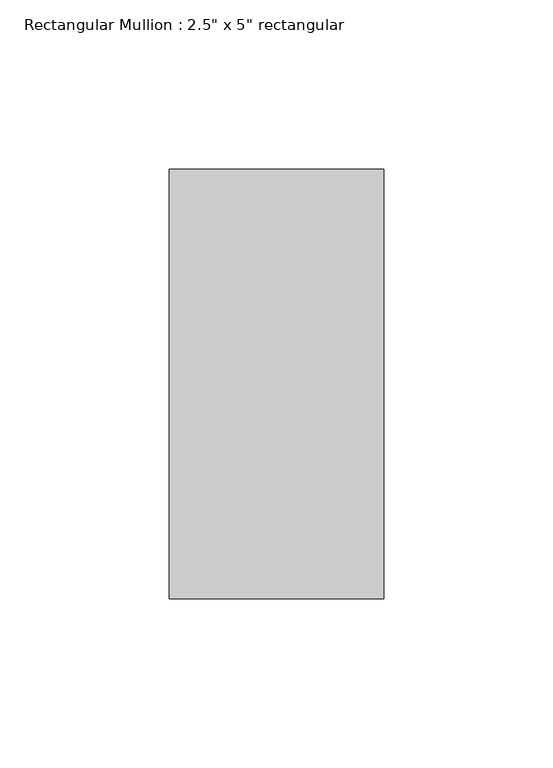
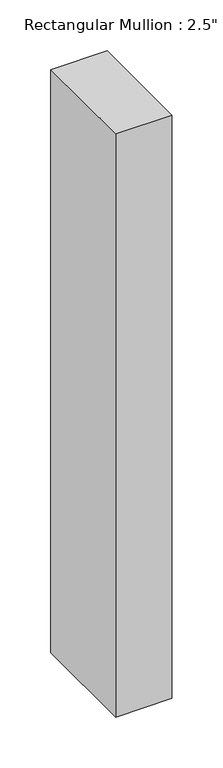
"""IFC4 building model written with IfcOpenShell, lengths in millimetres: member geometry."""

from ifc_helpers import new_model, si_unit, frame, origin, place, context, project, spatial, polyline, outline, extrude, source, transform, mapped, element, save


def member_b955a9e9(model_context):
    return source(origin(), model_context, "Body", "SweptSolid", [
        extrude(outline(polyline([(0.0, 63.5), (0.0, -63.5), (-63.5, -63.5), (-63.5, 63.5), (0.0, 63.5)])), frame((0.0, 0.0, -698.5), z_axis=(0.0, 0.0, 1.0), x_axis=(1.0, 0.0, 0.0)), (0.0, 0.0, 1.0), 698.5),
    ])


if __name__ == "__main__":
    model = new_model("IFC4")
    model_context = context("Model", 3, world=origin())
    ifc_project = project(units=[si_unit("LENGTHUNIT", "METRE", prefix="MILLI")], contexts=[model_context])
    site = spatial("IfcSite", under=ifc_project)
    building = spatial("IfcBuilding", under=site)
    placement = place(None, origin())
    member_shape = member_b955a9e9(model_context)
    element("IfcMember", 1, ObjectType="Rectangular Mullion : 2.5\" x 5\" rectangular", at=placement, inside=building, context=model_context, shape_type="MappedRepresentation", body=[
        mapped(member_shape, transform((0.0, 0.0, 0.0), x_axis=(1.0, 0.0, 0.0), y_axis=(0.0, 1.0, 0.0), z_axis=(0.0, 0.0, 1.0))),
    ])
    save(model, "model.ifc")

# Revit data of these elements
# Type "Rectangular Mullion : 2.5\" x 5\" rectangular"
#   built-in parameter 1007304 = 0.416667 (stored number, unit not read)
#   built-in parameter 1007301 = 0.104167 (stored number, unit not read)
#   built-in parameter 1007300 = 0.104167 (stored number, unit not read)
# Element 1 (IfcMember, "Rectangular Mullion : 2.5\" x 5\" rectangular")
#   Materials on its faces: "Aluminum"
# Materials
#   "Aluminum": class "Metal", colour RGB 247 247 247, transparency 0, Description = "Aluminum 6061", Cost = 0
